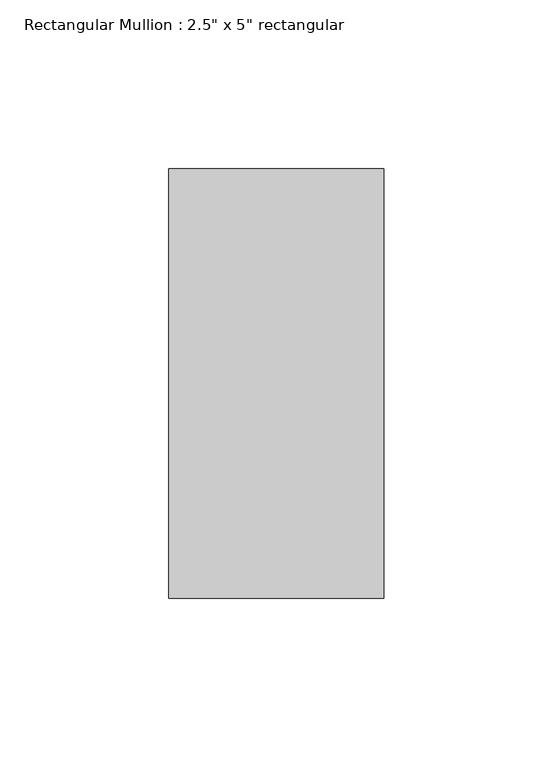
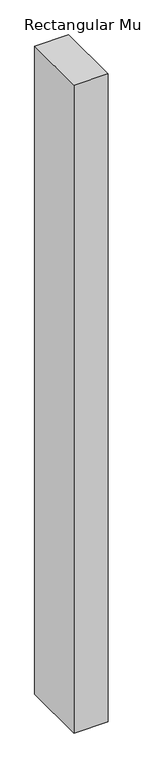
"""IFC4 building model written with IfcOpenShell, lengths in millimetres: member geometry."""

from ifc_helpers import new_model, si_unit, frame, origin, place, context, project, spatial, polyline, outline, extrude, source, transform, mapped, element, save


def member_cba00588(model_context):
    return source(origin(), model_context, "Body", "SweptSolid", [
        extrude(outline(polyline([(0.0, 63.5), (0.0, -63.5), (-63.5, -63.5), (-63.5, 63.5), (0.0, 63.5)])), frame((0.0, 0.0, -1276.35), z_axis=(0.0, 0.0, 1.0), x_axis=(1.0, 0.0, 0.0)), (0.0, 0.0, 1.0), 1276.35),
    ])


if __name__ == "__main__":
    model = new_model("IFC4")
    model_context = context("Model", 3, world=origin())
    ifc_project = project(units=[si_unit("LENGTHUNIT", "METRE", prefix="MILLI")], contexts=[model_context])
    site = spatial("IfcSite", under=ifc_project)
    building = spatial("IfcBuilding", under=site)
    placement = place(None, origin())
    member_shape = member_cba00588(model_context)
    element("IfcMember", 1, ObjectType="Rectangular Mullion : 2.5\" x 5\" rectangular", at=placement, inside=building, context=model_context, shape_type="MappedRepresentation", body=[
        mapped(member_shape, transform((0.0, 0.0, 0.0), x_axis=(1.0, 0.0, 0.0), y_axis=(0.0, 1.0, 0.0), z_axis=(0.0, 0.0, 1.0))),
    ])
    save(model, "model.ifc")

# Revit data of these elements
# Type "Rectangular Mullion : 2.5\" x 5\" rectangular"
#   built-in parameter 1007304 = 0.416667 (stored number, unit not read)
#   built-in parameter 1007301 = 0.104167 (stored number, unit not read)
#   built-in parameter 1007300 = 0.104167 (stored number, unit not read)
# Element 1 (IfcMember, "Rectangular Mullion : 2.5\" x 5\" rectangular")
#   Materials on its faces: "Aluminum"
# Materials
#   "Aluminum": class "Metal", colour RGB 247 247 247, transparency 0, Description = "Aluminum 6061", Cost = 0
